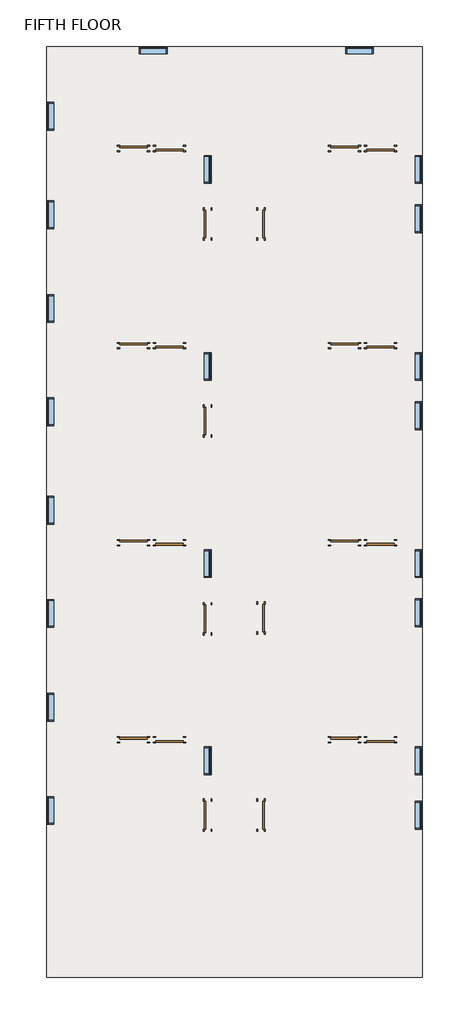
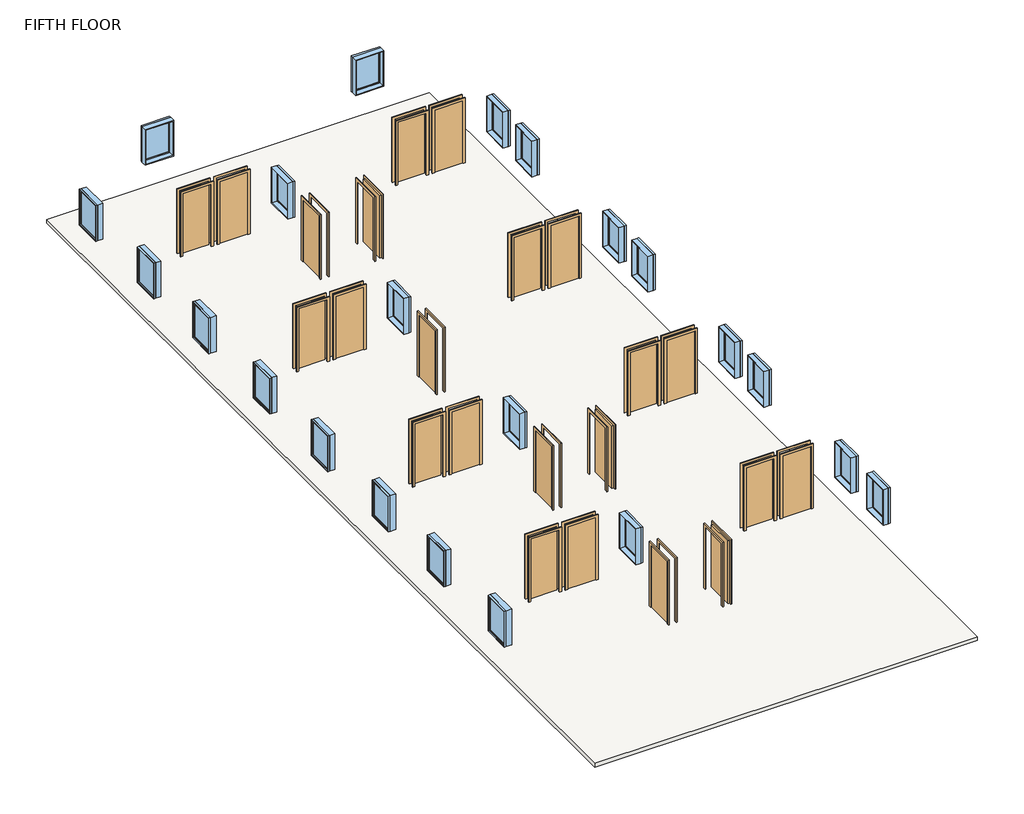
# One storey: 23 doors, 22 windows, 1 slab.
"""IFC4 building model written with IfcOpenShell, lengths in millimetres."""

from ifc_helpers import new_model, si_unit, frame, origin, place, context, project, spatial, polyline, outline, extrude, transform, mapped, element, save
from components import door_686f89d2, door_16372e1c, door_a90ba1ad, door_0ca8825f, window_c1f32544

model = new_model("IFC4")

# Units and contexts
model_context = context("Model", 3, world=origin())
ifc_project = project(units=[si_unit("LENGTHUNIT", "METRE", prefix="MILLI")], contexts=[model_context])

# Site, building, storey
site = spatial("IfcSite", under=ifc_project)
building = spatial("IfcBuilding", under=site)
storey = spatial("IfcBuildingStorey", under=building, Name="FIFTH FLOOR", Elevation=16002.0)

# Doors
placement = place(None, origin())
door_shape = door_686f89d2(model_context)
element("IfcDoor", 1, ObjectType="Single-Flush : 36\" x 84\"", at=placement, inside=storey, context=model_context, shape_type="MappedRepresentation", body=[
    mapped(door_shape, transform((-9863.5902461, 11952.2710592, 16002.0), x_axis=(-1.0, 0.0, 0.0), y_axis=(0.0, -1.0, 0.0), z_axis=(0.0, 0.0, 1.0))),
])
element("IfcDoor", 2, ObjectType="Single-Flush : 36\" x 84\"", at=placement, inside=storey, context=model_context, shape_type="MappedRepresentation", body=[
    mapped(door_shape, transform((-9863.5902461, 5475.2710592, 16002.0), x_axis=(-1.0, 0.0, 0.0), y_axis=(0.0, -1.0, 0.0), z_axis=(0.0, 0.0, 1.0))),
])
element("IfcDoor", 3, ObjectType="Single-Flush : 36\" x 84\"", at=placement, inside=storey, context=model_context, shape_type="MappedRepresentation", body=[
    mapped(door_shape, transform((-9863.5902461, -1001.7289408, 16002.0), x_axis=(-1.0, 0.0, 0.0), y_axis=(0.0, -1.0, 0.0), z_axis=(0.0, 0.0, 1.0))),
])
element("IfcDoor", 4, ObjectType="Single-Flush : 36\" x 84\"", at=placement, inside=storey, context=model_context, shape_type="MappedRepresentation", body=[
    mapped(door_shape, transform((-9863.5902461, -7478.7289408, 16002.0), x_axis=(-1.0, 0.0, 0.0), y_axis=(0.0, -1.0, 0.0), z_axis=(0.0, 0.0, 1.0))),
])
element("IfcDoor", 5, ObjectType="Single-Flush : 36\" x 84\"", at=placement, inside=storey, context=model_context, shape_type="MappedRepresentation", body=[
    mapped(door_shape, transform((-2929.3902461, -7478.7289408, 16002.0), x_axis=(-1.0, 0.0, 0.0), y_axis=(0.0, -1.0, 0.0), z_axis=(0.0, 0.0, 1.0))),
])
element("IfcDoor", 6, ObjectType="Single-Flush : 36\" x 84\"", at=placement, inside=storey, context=model_context, shape_type="MappedRepresentation", body=[
    mapped(door_shape, transform((-2929.3902461, -1001.7289408, 16002.0), x_axis=(-1.0, 0.0, 0.0), y_axis=(0.0, -1.0, 0.0), z_axis=(0.0, 0.0, 1.0))),
])
element("IfcDoor", 7, ObjectType="Single-Flush : 36\" x 84\"", at=placement, inside=storey, context=model_context, shape_type="MappedRepresentation", body=[
    mapped(door_shape, transform((-2929.3902461, 5475.2710592, 16002.0), x_axis=(-1.0, 0.0, 0.0), y_axis=(0.0, -1.0, 0.0), z_axis=(0.0, 0.0, 1.0))),
])
element("IfcDoor", 8, ObjectType="Single-Flush : 36\" x 84\"", at=placement, inside=storey, context=model_context, shape_type="MappedRepresentation", body=[
    mapped(door_shape, transform((-2929.3902461, 11952.2710592, 16002.0), x_axis=(-1.0, 0.0, 0.0), y_axis=(0.0, -1.0, 0.0), z_axis=(0.0, 0.0, 1.0))),
])
door_2_shape = door_16372e1c(model_context)
element("IfcDoor", 9, ObjectType="Single-Flush : 36\" x 84\"", at=placement, inside=storey, context=model_context, shape_type="MappedRepresentation", body=[
    mapped(door_2_shape, transform((-8682.4902461, 11952.2710592, 16002.0), x_axis=(-1.0, 0.0, 0.0), y_axis=(0.0, -1.0, 0.0), z_axis=(0.0, 0.0, 1.0))),
])
element("IfcDoor", 10, ObjectType="Single-Flush : 36\" x 84\"", at=placement, inside=storey, context=model_context, shape_type="MappedRepresentation", body=[
    mapped(door_2_shape, transform((-8682.4902461, 5475.2710592, 16002.0), x_axis=(-1.0, 0.0, 0.0), y_axis=(0.0, -1.0, 0.0), z_axis=(0.0, 0.0, 1.0))),
])
element("IfcDoor", 11, ObjectType="Single-Flush : 36\" x 84\"", at=placement, inside=storey, context=model_context, shape_type="MappedRepresentation", body=[
    mapped(door_2_shape, transform((-8682.4902461, -1001.7289408, 16002.0), x_axis=(-1.0, 0.0, 0.0), y_axis=(0.0, -1.0, 0.0), z_axis=(0.0, 0.0, 1.0))),
])
element("IfcDoor", 12, ObjectType="Single-Flush : 36\" x 84\"", at=placement, inside=storey, context=model_context, shape_type="MappedRepresentation", body=[
    mapped(door_2_shape, transform((-8682.4902461, -7478.7289408, 16002.0), x_axis=(-1.0, 0.0, 0.0), y_axis=(0.0, -1.0, 0.0), z_axis=(0.0, 0.0, 1.0))),
])
element("IfcDoor", 13, ObjectType="Single-Flush : 36\" x 84\"", at=placement, inside=storey, context=model_context, shape_type="MappedRepresentation", body=[
    mapped(door_2_shape, transform((-1748.2902461, -7478.7289408, 16002.0), x_axis=(-1.0, 0.0, 0.0), y_axis=(0.0, -1.0, 0.0), z_axis=(0.0, 0.0, 1.0))),
])
element("IfcDoor", 14, ObjectType="Single-Flush : 36\" x 84\"", at=placement, inside=storey, context=model_context, shape_type="MappedRepresentation", body=[
    mapped(door_2_shape, transform((-1748.2902461, -1001.7289408, 16002.0), x_axis=(-1.0, 0.0, 0.0), y_axis=(0.0, -1.0, 0.0), z_axis=(0.0, 0.0, 1.0))),
])
element("IfcDoor", 15, ObjectType="Single-Flush : 36\" x 84\"", at=placement, inside=storey, context=model_context, shape_type="MappedRepresentation", body=[
    mapped(door_2_shape, transform((-1748.2902461, 5475.2710592, 16002.0), x_axis=(-1.0, 0.0, 0.0), y_axis=(0.0, -1.0, 0.0), z_axis=(0.0, 0.0, 1.0))),
])
element("IfcDoor", 16, ObjectType="Single-Flush : 36\" x 84\"", at=placement, inside=storey, context=model_context, shape_type="MappedRepresentation", body=[
    mapped(door_2_shape, transform((-1748.2902461, 11952.2710592, 16002.0), x_axis=(-1.0, 0.0, 0.0), y_axis=(0.0, -1.0, 0.0), z_axis=(0.0, 0.0, 1.0))),
])
door_3_shape = door_a90ba1ad(model_context)
element("IfcDoor", 17, ObjectType="Single-Flush : 36\" x 84\"", at=placement, inside=storey, context=model_context, shape_type="MappedRepresentation", body=[
    mapped(door_3_shape, transform((-7425.1902461, 9475.7710592, 16002.0), x_axis=(0.0, -1.0, 0.0), y_axis=(1.0, 0.0, 0.0), z_axis=(0.0, 0.0, 1.0))),
])
element("IfcDoor", 18, ObjectType="Single-Flush : 36\" x 84\"", at=placement, inside=storey, context=model_context, shape_type="MappedRepresentation", body=[
    mapped(door_3_shape, transform((-7425.1902461, 2998.7710592, 16002.0), x_axis=(0.0, -1.0, 0.0), y_axis=(1.0, 0.0, 0.0), z_axis=(0.0, 0.0, 1.0))),
])
element("IfcDoor", 19, ObjectType="Single-Flush : 36\" x 84\"", at=placement, inside=storey, context=model_context, shape_type="MappedRepresentation", body=[
    mapped(door_3_shape, transform((-7425.1902461, -3503.6289408, 16002.0), x_axis=(0.0, -1.0, 0.0), y_axis=(1.0, 0.0, 0.0), z_axis=(0.0, 0.0, 1.0))),
])
element("IfcDoor", 20, ObjectType="Single-Flush : 36\" x 84\"", at=placement, inside=storey, context=model_context, shape_type="MappedRepresentation", body=[
    mapped(door_3_shape, transform((-7425.1902461, -9955.2289408, 16002.0), x_axis=(0.0, -1.0, 0.0), y_axis=(1.0, 0.0, 0.0), z_axis=(0.0, 0.0, 1.0))),
])
door_4_shape = door_0ca8825f(model_context)
element("IfcDoor", 21, ObjectType="Single-Flush : 36\" x 84\"", at=placement, inside=storey, context=model_context, shape_type="MappedRepresentation", body=[
    mapped(door_4_shape, transform((-5672.5902461, 9475.7710592, 16002.0), x_axis=(0.0, -1.0, 0.0), y_axis=(1.0, 0.0, 0.0), z_axis=(0.0, 0.0, 1.0))),
])
element("IfcDoor", 22, ObjectType="Single-Flush : 36\" x 84\"", at=placement, inside=storey, context=model_context, shape_type="MappedRepresentation", body=[
    mapped(door_4_shape, transform((-5672.5902461, -3478.2289408, 16002.0), x_axis=(0.0, -1.0, 0.0), y_axis=(1.0, 0.0, 0.0), z_axis=(0.0, 0.0, 1.0))),
])
element("IfcDoor", 23, ObjectType="Single-Flush : 36\" x 84\"", at=placement, inside=storey, context=model_context, shape_type="MappedRepresentation", body=[
    mapped(door_4_shape, transform((-5672.5902461, -9955.2289408, 16002.0), x_axis=(0.0, -1.0, 0.0), y_axis=(1.0, 0.0, 0.0), z_axis=(0.0, 0.0, 1.0))),
])

# Slab
element("IfcSlab", 24, ObjectType="Generic - 12\"", at=placement, inside=storey, context=model_context, shape_type="SweptSolid", body=[
    extrude(outline(polyline([(-376.6902461, 15305.0710592), (-376.6902461, -15289.2289408), (-12721.0902461, -15289.2289408), (-12721.0902461, 15305.0710592), (-376.6902461, 15305.0710592)])), frame((0.0, 0.0, 15875.0), z_axis=(0.0, 0.0, 1.0), x_axis=(1.0, 0.0, 0.0)), (0.0, 0.0, 1.0), 127.0),
])

# Windows
window_shape = window_c1f32544(model_context)
element("IfcWindow", 25, ObjectType="Fixed : 36\" x 48\"", at=placement, inside=storey, context=model_context, shape_type="MappedRepresentation", body=[
    mapped(window_shape, transform((-9177.7902461, 15190.7710592, 16002.0), x_axis=(1.0, 0.0, 0.0), y_axis=(0.0, 1.0, 0.0), z_axis=(0.0, 0.0, 1.0))),
])
element("IfcWindow", 26, ObjectType="Fixed : 36\" x 48\"", at=placement, inside=storey, context=model_context, shape_type="MappedRepresentation", body=[
    mapped(window_shape, transform((-2395.9902461, 15190.7710592, 16002.0), x_axis=(1.0, 0.0, 0.0), y_axis=(0.0, 1.0, 0.0), z_axis=(0.0, 0.0, 1.0))),
])
element("IfcWindow", 27, ObjectType="Fixed : 36\" x 48\"", at=placement, inside=storey, context=model_context, shape_type="MappedRepresentation", body=[
    mapped(window_shape, transform((-490.9902461, 11228.3710592, 16002.0), x_axis=(0.0, -1.0, 0.0), y_axis=(1.0, 0.0, 0.0), z_axis=(0.0, 0.0, 1.0))),
])
element("IfcWindow", 28, ObjectType="Fixed : 36\" x 48\"", at=placement, inside=storey, context=model_context, shape_type="MappedRepresentation", body=[
    mapped(window_shape, transform((-490.9902461, 9609.1210592, 16002.0), x_axis=(0.0, -1.0, 0.0), y_axis=(1.0, 0.0, 0.0), z_axis=(0.0, 0.0, 1.0))),
])
element("IfcWindow", 29, ObjectType="Fixed : 36\" x 48\"", at=placement, inside=storey, context=model_context, shape_type="MappedRepresentation", body=[
    mapped(window_shape, transform((-490.9902461, 4751.3710592, 16002.0), x_axis=(0.0, -1.0, 0.0), y_axis=(1.0, 0.0, 0.0), z_axis=(0.0, 0.0, 1.0))),
])
element("IfcWindow", 30, ObjectType="Fixed : 36\" x 48\"", at=placement, inside=storey, context=model_context, shape_type="MappedRepresentation", body=[
    mapped(window_shape, transform((-490.9902461, 3132.1210592, 16002.0), x_axis=(0.0, -1.0, 0.0), y_axis=(1.0, 0.0, 0.0), z_axis=(0.0, 0.0, 1.0))),
])
element("IfcWindow", 31, ObjectType="Fixed : 36\" x 48\"", at=placement, inside=storey, context=model_context, shape_type="MappedRepresentation", body=[
    mapped(window_shape, transform((-490.9902461, -1725.6289408, 16002.0), x_axis=(0.0, -1.0, 0.0), y_axis=(1.0, 0.0, 0.0), z_axis=(0.0, 0.0, 1.0))),
])
element("IfcWindow", 32, ObjectType="Fixed : 36\" x 48\"", at=placement, inside=storey, context=model_context, shape_type="MappedRepresentation", body=[
    mapped(window_shape, transform((-490.9902461, -3344.8789408, 16002.0), x_axis=(0.0, -1.0, 0.0), y_axis=(1.0, 0.0, 0.0), z_axis=(0.0, 0.0, 1.0))),
])
element("IfcWindow", 33, ObjectType="Fixed : 36\" x 48\"", at=placement, inside=storey, context=model_context, shape_type="MappedRepresentation", body=[
    mapped(window_shape, transform((-490.9902461, -8202.6289408, 16002.0), x_axis=(0.0, -1.0, 0.0), y_axis=(1.0, 0.0, 0.0), z_axis=(0.0, 0.0, 1.0))),
])
element("IfcWindow", 34, ObjectType="Fixed : 36\" x 48\"", at=placement, inside=storey, context=model_context, shape_type="MappedRepresentation", body=[
    mapped(window_shape, transform((-490.9902461, -9993.3289408, 16002.0), x_axis=(0.0, -1.0, 0.0), y_axis=(1.0, 0.0, 0.0), z_axis=(0.0, 0.0, 1.0))),
])
element("IfcWindow", 35, ObjectType="Fixed : 36\" x 48\"", at=placement, inside=storey, context=model_context, shape_type="MappedRepresentation", body=[
    mapped(window_shape, transform((-7425.1902461, -8202.6289408, 16002.0), x_axis=(0.0, -1.0, 0.0), y_axis=(1.0, 0.0, 0.0), z_axis=(0.0, 0.0, 1.0))),
])
element("IfcWindow", 36, ObjectType="Fixed : 36\" x 48\"", at=placement, inside=storey, context=model_context, shape_type="MappedRepresentation", body=[
    mapped(window_shape, transform((-7425.1902461, -1725.6289408, 16002.0), x_axis=(0.0, -1.0, 0.0), y_axis=(1.0, 0.0, 0.0), z_axis=(0.0, 0.0, 1.0))),
])
element("IfcWindow", 37, ObjectType="Fixed : 36\" x 48\"", at=placement, inside=storey, context=model_context, shape_type="MappedRepresentation", body=[
    mapped(window_shape, transform((-7425.1902461, 4751.3710592, 16002.0), x_axis=(0.0, -1.0, 0.0), y_axis=(1.0, 0.0, 0.0), z_axis=(0.0, 0.0, 1.0))),
])
element("IfcWindow", 38, ObjectType="Fixed : 36\" x 48\"", at=placement, inside=storey, context=model_context, shape_type="MappedRepresentation", body=[
    mapped(window_shape, transform((-7425.1902461, 11228.3710592, 16002.0), x_axis=(0.0, -1.0, 0.0), y_axis=(1.0, 0.0, 0.0), z_axis=(0.0, 0.0, 1.0))),
])
element("IfcWindow", 39, ObjectType="Fixed : 36\" x 48\"", at=placement, inside=storey, context=model_context, shape_type="MappedRepresentation", body=[
    mapped(window_shape, transform((-12606.7902461, 13057.1710592, 16002.0), x_axis=(0.0, 1.0, 0.0), y_axis=(-1.0, 0.0, 0.0), z_axis=(0.0, 0.0, 1.0))),
])
element("IfcWindow", 40, ObjectType="Fixed : 36\" x 48\"", at=placement, inside=storey, context=model_context, shape_type="MappedRepresentation", body=[
    mapped(window_shape, transform((-12606.7902461, 9818.6710592, 16002.0), x_axis=(0.0, 1.0, 0.0), y_axis=(-1.0, 0.0, 0.0), z_axis=(0.0, 0.0, 1.0))),
])
element("IfcWindow", 41, ObjectType="Fixed : 36\" x 48\"", at=placement, inside=storey, context=model_context, shape_type="MappedRepresentation", body=[
    mapped(window_shape, transform((-12606.7902461, 6732.5710592, 16002.0), x_axis=(0.0, 1.0, 0.0), y_axis=(-1.0, 0.0, 0.0), z_axis=(0.0, 0.0, 1.0))),
])
element("IfcWindow", 42, ObjectType="Fixed : 36\" x 48\"", at=placement, inside=storey, context=model_context, shape_type="MappedRepresentation", body=[
    mapped(window_shape, transform((-12606.7902461, 3341.6710592, 16002.0), x_axis=(0.0, 1.0, 0.0), y_axis=(-1.0, 0.0, 0.0), z_axis=(0.0, 0.0, 1.0))),
])
element("IfcWindow", 43, ObjectType="Fixed : 36\" x 48\"", at=placement, inside=storey, context=model_context, shape_type="MappedRepresentation", body=[
    mapped(window_shape, transform((-12606.7902461, 103.1710592, 16002.0), x_axis=(0.0, 1.0, 0.0), y_axis=(-1.0, 0.0, 0.0), z_axis=(0.0, 0.0, 1.0))),
])
element("IfcWindow", 44, ObjectType="Fixed : 36\" x 48\"", at=placement, inside=storey, context=model_context, shape_type="MappedRepresentation", body=[
    mapped(window_shape, transform((-12606.7902461, -3287.7289408, 16002.0), x_axis=(0.0, 1.0, 0.0), y_axis=(-1.0, 0.0, 0.0), z_axis=(0.0, 0.0, 1.0))),
])
element("IfcWindow", 45, ObjectType="Fixed : 36\" x 48\"", at=placement, inside=storey, context=model_context, shape_type="MappedRepresentation", body=[
    mapped(window_shape, transform((-12606.7902461, -6373.8289408, 16002.0), x_axis=(0.0, 1.0, 0.0), y_axis=(-1.0, 0.0, 0.0), z_axis=(0.0, 0.0, 1.0))),
])
element("IfcWindow", 46, ObjectType="Fixed : 36\" x 48\"", at=placement, inside=storey, context=model_context, shape_type="MappedRepresentation", body=[
    mapped(window_shape, transform((-12606.7902461, -9764.7289408, 16002.0), x_axis=(0.0, 1.0, 0.0), y_axis=(-1.0, 0.0, 0.0), z_axis=(0.0, 0.0, 1.0))),
])

save(model, "model.ifc")

# Revit data of these elements
# Type "Single-Flush : 36\" x 84\""
#   Type Mark = "1"
#   Construction Type Id = "MDOOR"
#   Assembly Code = "C1020"
#   Analytic Construction = "Metal"
#   Thickness = 0' - 2"
#   Heat Transfer Coefficient (U) = 0.651978 BTU/(h·ft²·°F)
#   Height = 7' - 0"
#   Trim Projection Ext = 0' - 1"
#   Trim Projection Int = 0' - 1"
#   Trim Width = 0' - 3"
#   Width = 3' - 0"
#   Define Thermal Properties by = 1
#   Door Material = Door - Panel
#   Frame Material = Door - Frame
#   Visual Light Transmittance = 0
#   Solar Heat Gain Coefficient = 0
#   Function = (empty or 0)
#   Wall Closure = (empty or 0)
# Type "Generic - 12\""
#   Assembly Code = "B1010"
#   Function = 0
#   Layers, outside or top first: 0' - 5" no material (function 1)
# Type "Fixed : 36\" x 48\""
#   Type Mark = "1"
#   Construction Type Id = "GSP4R"
#   Assembly Code = "B2020100"
#   Analytic Construction = "1/8 in Pilkington single glazing"
#   Visual Light Transmittance = 0.9
#   Solar Heat Gain Coefficient = 0.78
#   Heat Transfer Coefficient (U) = 0.6496 BTU/(h·ft²·°F)
#   Height = 4' - 0"
#   Default Sill Height = 3' - 0"
#   Width = 3' - 0"
#   Window Inset = 0' - 0 3/4"
#   Define Thermal Properties by = 1
#   Glass Pane Material = Glass
#   Sash Material = Sash
#   Wall Closure = (empty or 0)
# Elements 1, 2, 3, 4, 5, 6, 7, 8, 9, 10, 11, 12, 13, 14, 15, 16, 17, 18, 19, 20, 21, 22, 23 (IfcDoor, "Single-Flush : 36\" x 84\"")
#   Phase Created = New Construction
#   Materials on its faces: "Door - Frame", "Door - Panel"
# Element 24 (IfcSlab, "Generic - 12\"")
#   Height Offset From Level = 0' - 0"
#   Phase Created = New Construction
#   Materials on its faces: "Default Floor"
# Element 25 (IfcWindow, "Fixed : 36\" x 48\"")
#   Mark = "117"
#   Phase Created = New Construction
#   Materials on its faces: "Sash", "Glass"
# Element 26 (IfcWindow, "Fixed : 36\" x 48\"")
#   Mark = "118"
#   Phase Created = New Construction
#   Materials on its faces: "Sash", "Glass"
# Element 27 (IfcWindow, "Fixed : 36\" x 48\"")
#   Mark = "119"
#   Phase Created = New Construction
#   Materials on its faces: "Sash", "Glass"
# Element 28 (IfcWindow, "Fixed : 36\" x 48\"")
#   Mark = "120"
#   Phase Created = New Construction
#   Materials on its faces: "Sash", "Glass"
# Element 29 (IfcWindow, "Fixed : 36\" x 48\"")
#   Mark = "121"
#   Phase Created = New Construction
#   Materials on its faces: "Sash", "Glass"
# Element 30 (IfcWindow, "Fixed : 36\" x 48\"")
#   Mark = "122"
#   Phase Created = New Construction
#   Materials on its faces: "Sash", "Glass"
# Element 31 (IfcWindow, "Fixed : 36\" x 48\"")
#   Mark = "123"
#   Phase Created = New Construction
#   Materials on its faces: "Sash", "Glass"
# Element 32 (IfcWindow, "Fixed : 36\" x 48\"")
#   Mark = "124"
#   Phase Created = New Construction
#   Materials on its faces: "Sash", "Glass"
# Element 33 (IfcWindow, "Fixed : 36\" x 48\"")
#   Mark = "125"
#   Phase Created = New Construction
#   Materials on its faces: "Sash", "Glass"
# Element 34 (IfcWindow, "Fixed : 36\" x 48\"")
#   Mark = "126"
#   Phase Created = New Construction
#   Materials on its faces: "Sash", "Glass"
# Element 35 (IfcWindow, "Fixed : 36\" x 48\"")
#   Mark = "127"
#   Phase Created = New Construction
#   Materials on its faces: "Sash", "Glass"
# Element 36 (IfcWindow, "Fixed : 36\" x 48\"")
#   Mark = "128"
#   Phase Created = New Construction
#   Materials on its faces: "Sash", "Glass"
# Element 37 (IfcWindow, "Fixed : 36\" x 48\"")
#   Mark = "129"
#   Phase Created = New Construction
#   Materials on its faces: "Sash", "Glass"
# Element 38 (IfcWindow, "Fixed : 36\" x 48\"")
#   Mark = "130"
#   Phase Created = New Construction
#   Materials on its faces: "Sash", "Glass"
# Element 39 (IfcWindow, "Fixed : 36\" x 48\"")
#   Mark = "131"
#   Phase Created = New Construction
#   Materials on its faces: "Sash", "Glass"
# Element 40 (IfcWindow, "Fixed : 36\" x 48\"")
#   Mark = "132"
#   Phase Created = New Construction
#   Materials on its faces: "Sash", "Glass"
# Element 41 (IfcWindow, "Fixed : 36\" x 48\"")
#   Mark = "133"
#   Phase Created = New Construction
#   Materials on its faces: "Sash", "Glass"
# Element 42 (IfcWindow, "Fixed : 36\" x 48\"")
#   Mark = "134"
#   Phase Created = New Construction
#   Materials on its faces: "Sash", "Glass"
# Element 43 (IfcWindow, "Fixed : 36\" x 48\"")
#   Mark = "135"
#   Phase Created = New Construction
#   Materials on its faces: "Sash", "Glass"
# Element 44 (IfcWindow, "Fixed : 36\" x 48\"")
#   Mark = "136"
#   Phase Created = New Construction
#   Materials on its faces: "Sash", "Glass"
# Element 45 (IfcWindow, "Fixed : 36\" x 48\"")
#   Mark = "137"
#   Phase Created = New Construction
#   Materials on its faces: "Sash", "Glass"
# Element 46 (IfcWindow, "Fixed : 36\" x 48\"")
#   Mark = "138"
#   Phase Created = New Construction
#   Materials on its faces: "Sash", "Glass"
# Materials
#   "Door - Panel": class "Wood", colour RGB 210 159 95, transparency 0
#   "Door - Frame": colour RGB 118 70 51, transparency 0
#   "Glass": class "Glass", colour RGB 0 128 192, transparency 0.75, Description = "Soda Lime Glass", Cost = 0
#   "Sash": class "Wood", colour RGB 224 178 126, transparency 0
#   "Default Floor": colour RGB 128 128 128, transparency 0
